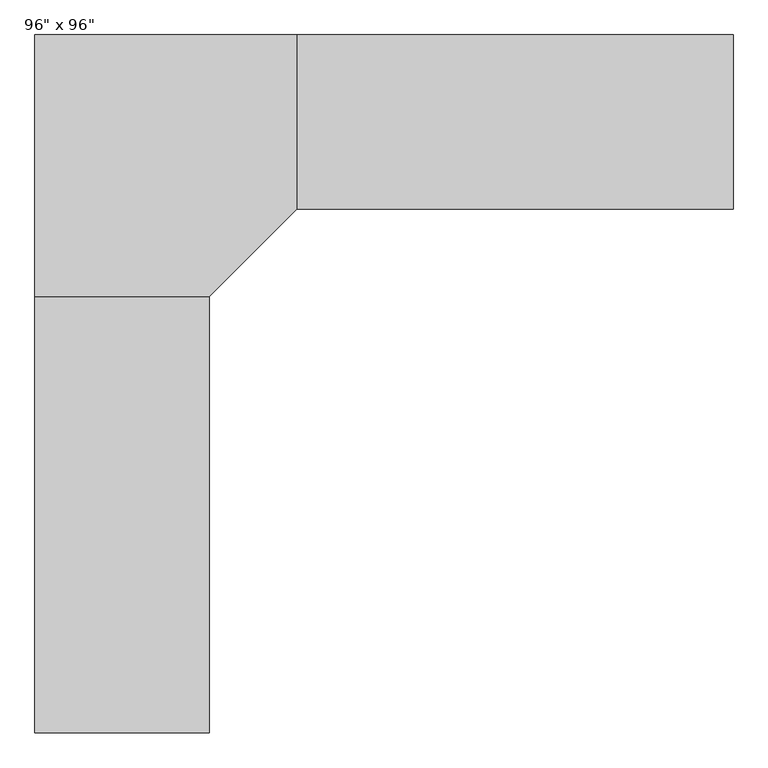
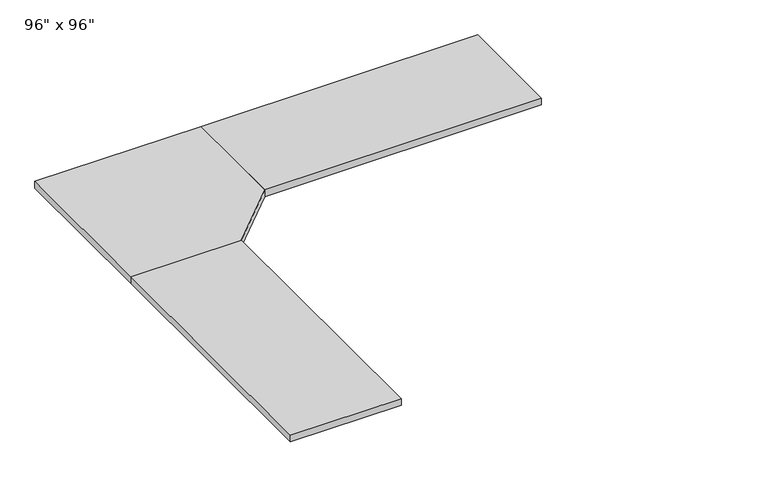
"""IFC4 building model written with IfcOpenShell, lengths in millimetres: furniture geometry."""

from ifc_helpers import new_model, si_unit, frame, origin, place, context, project, spatial, polyline, outline, extrude, source, transform, mapped, element, save


def furniture_07436f11(model_context):
    return source(origin(), model_context, "Body", "SweptSolid", [
        extrude(outline(polyline([(-80.9317522, -545.8230076), (833.4682478, -545.8230076), (833.4682478, -1155.4230076), (528.6682478, -1460.2230076), (-80.9317522, -1460.2230076), (-80.9317522, -545.8230076)])), frame((0.0, 0.0, 723.9), z_axis=(0.0, 0.0, 1.0), x_axis=(1.0, 0.0, 0.0)), (0.0, 0.0, 1.0), 38.1),
        extrude(outline(polyline([(528.6682478, -2984.2230076), (-80.9317522, -2984.2230076), (-80.9317522, -1460.2230076), (528.6682478, -1460.2230076), (528.6682478, -2984.2230076)])), frame((0.0, 0.0, 723.9), z_axis=(0.0, 0.0, 1.0), x_axis=(1.0, 0.0, 0.0)), (0.0, 0.0, 1.0), 38.1),
        extrude(outline(polyline([(2357.4682478, -1155.4230076), (833.4682478, -1155.4230076), (833.4682478, -545.8230076), (2357.4682478, -545.8230076), (2357.4682478, -1155.4230076)])), frame((0.0, 0.0, 723.9), z_axis=(0.0, 0.0, 1.0), x_axis=(1.0, 0.0, 0.0)), (0.0, 0.0, 1.0), 38.1),
    ])


if __name__ == "__main__":
    model = new_model("IFC4")
    model_context = context("Model", 3, world=origin())
    ifc_project = project(units=[si_unit("LENGTHUNIT", "METRE", prefix="MILLI")], contexts=[model_context])
    site = spatial("IfcSite", under=ifc_project)
    building = spatial("IfcBuilding", under=site)
    placement = place(None, origin())
    furniture_shape = furniture_07436f11(model_context)
    element("IfcFurniture", 1, ObjectType="96\" x 96\"", at=placement, inside=building, context=model_context, shape_type="MappedRepresentation", body=[
        mapped(furniture_shape, transform((0.0, 0.0, 0.0), x_axis=(1.0, 0.0, 0.0), y_axis=(0.0, 1.0, 0.0), z_axis=(0.0, 0.0, 1.0))),
    ])
    save(model, "model.ifc")

# Revit data of these elements
# Type "96\" x 96\""
#   Assembly Code = "E2020"
#   Desktop Height = 2' - 6"
#   Desktop1 Width = 2' - 0"
#   Desktop2 Width = 2' - 0"
#   Panel1 Length = 5' - 0"
#   Panel2 Length = 5' - 0"
#   Work Top Material = Laminate, Ivory, Matte
# Element 1 (IfcFurniture, "96\" x 96\"")
#   Materials on its faces: "Laminate, Ivory, Matte"
# Materials
#   "Laminate, Ivory, Matte": class "Plastic", colour RGB 247 247 239, transparency 0, Description = "Plastic Laminate - Ivory, Matte", Cost = 0
